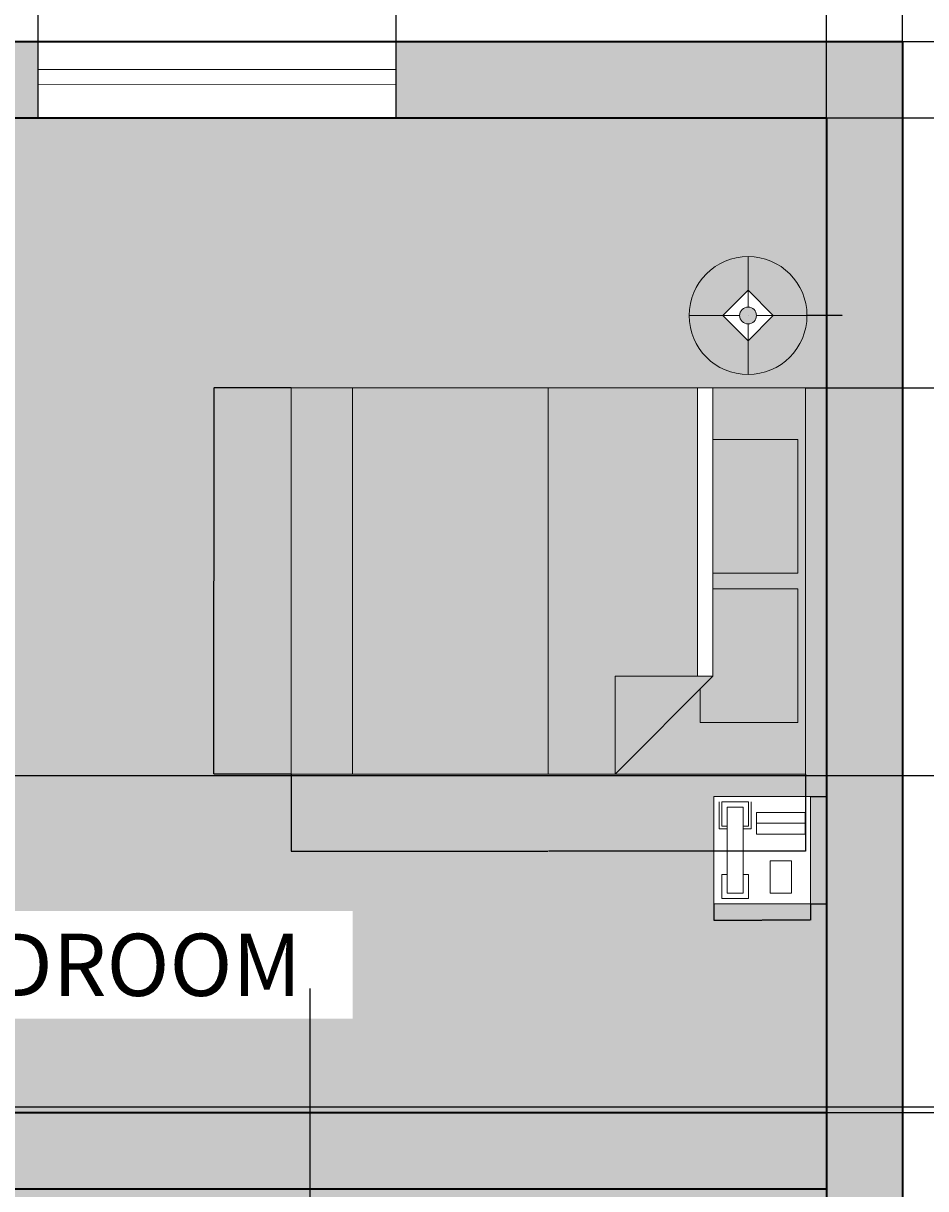
# Model space of a CAD drawing. Units: millimetres. Extents: x -229 to 16545, y -10488 to 4272.
# Tile 27 of 29: x 11362 to 14086, y -1208 to 2307. Entities that reach past the tile are written whole.
import ezdxf

# ---------------------------------------------------------------- set-up
doc = ezdxf.new("R2010")
doc.units = ezdxf.units.MM
for name, color, linetype, lineweight in [('A-ANNO-DIMS', 2, 'Continuous', 18), ('A-AREA-IDEN', 7, 'Continuous', 18), ('A-FURN', 8, 'Continuous', 18), ('A-FURN-PATT', 252, 'Continuous', 13), ('A-GLAZ', 4, 'Continuous', 18), ('A-WALL', 7, 'Continuous', 35)]:
    doc.layers.add(name, color=color, linetype=linetype, lineweight=lineweight)
doc.layers.add('A-FLOR-PATT', color=254, linetype='Continuous', lineweight=13, true_color=0xfeeab9)
doc.layers.add('A-WALL-PATT', color=18, linetype='Continuous', lineweight=13, true_color=0x000000)
doc.styles.get("Standard").update_dxf_attribs({"font": 'arial.ttf'})
doc.dimstyles.get("Standard").update_dxf_attribs({"dimtxt": 0.18, "dimasz": 0.18, "dimexe": 0.18, "dimexo": 0.0625, "dimgap": 0.09, "dimtad": 0, "dimtih": 1, "dimtoh": 1, "dimdec": 4, "dimzin": 0, "dimdsep": 46, "dimtxsty": 'Standard', "dimcen": 0.09, "dimadec": 0, "dimazin": 0, "dimtfac": 1, "dimtdec": 4, "dimtofl": 0, "dimtmove": 0, "dimatfit": 3, "dimfxl": 1, "dimtolj": 1, "dimtzin": 0, "dimarcsym": 0})

# ---------------------------------------------------------------- blocks, each defined once
blk = doc.blocks.new('Bed - Queen')
for p, q in [((0, -80.00003), (0, 0)), ((0, 0), (59.99999, 0)), ((59.99999, 0), (59.99999, -80.00003)), ((7.99999, -1.2), (28.79998, -1.2)), ((7.99999, -14.4), (7.99999, -1.2)), ((28.79998, -1.2), (28.79998, -14.4)), ((31.19999, -1.2), (51.99999, -1.2)), ((31.19999, -14.4), (31.19999, -1.2)), ((51.99999, -1.2), (51.99999, -16.4)), ((0, -14.4), (44.8, -14.4)), ((59.99999, -29.6), (44.8, -14.4)), ((44.8, -14.4), (44.8, -29.6)), ((44.8, -16.8), (0, -16.8)), ((51.99999, -16.4), (46.79936, -16.4)), ((44.8, -29.6), (59.99999, -29.6)), ((59.99999, -80.00003), (0, -80.00003))]:
    blk.add_line(p, q)
blk = doc.blocks.new('Lamp - Table')
for p, q in [((0, 7), (0, 1)), ((0, 3), (-3, 0)), ((3, 0), (0, 3)), ((-1, 0), (-7, 0)), ((-3, 0), (0, -3)), ((0, -3), (3, 0)), ((1, 0), (7, 0)), ((0, -1), (0, -7))]:
    blk.add_line(p, q)
for radius in [7, 1]:
    blk.add_circle((0, 0), radius)
blk = doc.blocks.new('Phone - Desk')
for p, q in [((-4.5, -5), (-4.5, 5)), ((-4.5, 5), (4.5, 5)), ((-4, 4.5), (-4, 2)), ((-3.75, 4.5), (-3.75, 2.25)), ((-1.25, 4.5), (-3.75, 4.5)), ((-1.25, 2.25), (-1.25, 4.5)), ((-1, 2), (-1, 4.5)), ((4.5, 5), (4.5, -5)), ((-3.25, 4), (-3.25, -4)), ((-3.25, 4), (-1.75, 4)), ((-1.75, -4), (-1.75, 4)), ((4, 3.5), (-0.5, 3.5)), ((-0.5, 3.5), (-0.5, 1.5)), ((4, 1.5), (4, 3.5)), ((-3.75, 2.25), (-3.25, 2.25)), ((-1.75, 2.25), (-1.25, 2.25)), ((-0.5, 2.5), (4, 2.5)), ((-4, 2), (-3.25, 2)), ((-1.75, 2), (-1, 2)), ((-0.5, 1.5), (4, 1.5)), ((2.75, -1), (0.75, -1)), ((0.75, -1), (0.75, -4)), ((2.75, -4), (2.75, -1)), ((-3.75, -2.25), (-3.25, -2.25)), ((-3.75, -4.5), (-3.75, -2.25)), ((-1.75, -2.25), (-1.25, -2.25)), ((-1.25, -2.25), (-1.25, -4.5)), ((-3.25, -4), (-1.75, -4)), ((0.75, -4), (2.75, -4)), ((4.5, -5), (-4.5, -5)), ((-1.25, -4.5), (-3.75, -4.5))]:
    blk.add_line(p, q)
blk = doc.blocks.new('*D31')
at = {"layer": 'A-ANNO-DIMS', "color": 0, "lineweight": -2, "transparency": 16777216}
for p, q in [((12170.5, 42.3), (12170.5, -190.7)), ((13722.9, 42.3), (13722.9, -190.7)), ((12170.6, -190.5), (12945.5, -190.5)), ((13722.7, -190.5), (12947.8, -190.5))]:
    blk.add_line(p, q, dxfattribs=at)
at = {"layer": 'A-ANNO-DIMS', "color": 0, "transparency": 16777216}
for points in [[(12170.6, -190.5), (12170.6, -190.5), (12170.5, -190.5)], [(13722.7, -190.5), (13722.7, -190.5), (13722.9, -190.5)]]:
    blk.add_solid(points, dxfattribs=at)
at = {"layer": 'Defpoints', "color": 0, "transparency": 16777216}
for p in [(12170.5, 42.4), (13722.9, 42.4), (13722.9, -190.5)]:
    blk.add_point(p, dxfattribs=at)
at = {"layer": 'A-ANNO-DIMS', "color": 0, "transparency": 16777216, "insert": (12946.7, -190.5), "char_height": 0.18, "attachment_point": 5}
blk.add_mtext('\\A1;QUEEN BED 1552', dxfattribs=at)
blk = doc.blocks.new('*D32')
at = {"layer": 'A-ANNO-DIMS', "color": 0, "lineweight": -2, "transparency": 16777216}
for p, q in [((12170.4, 1206.7), (11937.4, 1206.7)), ((11937.6, 1206.5), (11937.6, 624.7)), ((11937.6, 42.6), (11937.6, 624.4)), ((12170.4, 42.4), (11937.4, 42.4))]:
    blk.add_line(p, q, dxfattribs=at)
at = {"layer": 'A-ANNO-DIMS', "color": 0, "transparency": 16777216}
for points in [[(11937.6, 1206.5), (11937.6, 1206.5), (11937.6, 1206.7)], [(11937.6, 42.6), (11937.6, 42.6), (11937.6, 42.4)]]:
    blk.add_solid(points, dxfattribs=at)
at = {"layer": 'Defpoints', "color": 0, "transparency": 16777216}
for p in [(12170.5, 1206.7), (11937.6, 42.4), (12170.5, 42.4)]:
    blk.add_point(p, dxfattribs=at)
at = {"layer": 'A-ANNO-DIMS', "color": 0, "transparency": 16777216, "insert": (11937.6, 624.5), "char_height": 0.18, "attachment_point": 5}
blk.add_mtext('\\A1;1164', dxfattribs=at)
blk = doc.blocks.new('*D33')
at = {"layer": 'A-ANNO-DIMS', "color": 0, "lineweight": -2, "transparency": 16777216}
for p, q in [((13737.9, -25.2), (13786.6, -25.2)), ((13786.5, -25.4), (13786.5, -187.2)), ((13786.5, -349.4), (13786.5, -187.6)), ((13737.9, -349.6), (13786.6, -349.6))]:
    blk.add_line(p, q, dxfattribs=at)
at = {"layer": 'A-ANNO-DIMS', "color": 0, "transparency": 16777216}
for points in [[(13786.4, -25.4), (13786.5, -25.4), (13786.5, -25.2)], [(13786.4, -349.4), (13786.5, -349.4), (13786.5, -349.6)]]:
    blk.add_solid(points, dxfattribs=at)
at = {"layer": 'Defpoints', "color": 0, "transparency": 16777216}
for p in [(13737.8, -25.2), (13786.5, -25.2), (13737.8, -349.6)]:
    blk.add_point(p, dxfattribs=at)
at = {"layer": 'A-ANNO-DIMS', "color": 0, "transparency": 16777216, "insert": (13786.5, -187.4), "char_height": 0.18, "attachment_point": 5}
blk.add_mtext('\\A1;PHONE 324', dxfattribs=at)
blk = doc.blocks.new('*D34')
at = {"layer": 'A-ANNO-DIMS', "color": 0, "lineweight": -2, "transparency": 16777216}
for p, q in [((13445.9, -349.6), (13445.9, -398.4)), ((13737.8, -349.6), (13737.8, -398.4)), ((13446.1, -398.2), (13591.6, -398.2)), ((13737.6, -398.2), (13592.1, -398.2))]:
    blk.add_line(p, q, dxfattribs=at)
at = {"layer": 'A-ANNO-DIMS', "color": 0, "transparency": 16777216}
for points in [[(13446.1, -398.2), (13446.1, -398.3), (13445.9, -398.2)], [(13737.6, -398.2), (13737.6, -398.3), (13737.8, -398.2)]]:
    blk.add_solid(points, dxfattribs=at)
at = {"layer": 'Defpoints', "color": 0, "transparency": 16777216}
for p in [(13445.9, -349.6), (13737.8, -349.6), (13737.8, -398.2)]:
    blk.add_point(p, dxfattribs=at)
at = {"layer": 'A-ANNO-DIMS', "color": 0, "transparency": 16777216, "insert": (13591.8, -398.2), "char_height": 0.18, "attachment_point": 5}
blk.add_mtext('\\A1;292', dxfattribs=at)
blk = doc.blocks.new('*D45')
at = {"layer": 'A-ANNO-DIMS', "color": 0, "lineweight": -2, "transparency": 16777216}
for p, q in [((2015.9, 2251.8), (2015.9, 4271.7)), ((2016.1, 4271.5), (8015.5, 4271.5)), ((14015.8, 4271.5), (8016.4, 4271.5)), ((14015.9, 2251.8), (14015.9, 4271.7))]:
    blk.add_line(p, q, dxfattribs=at)
at = {"layer": 'A-ANNO-DIMS', "color": 0, "transparency": 16777216}
for points in [[(2016.1, 4271.5), (2016.1, 4271.4), (2015.9, 4271.5)], [(14015.8, 4271.5), (14015.8, 4271.4), (14015.9, 4271.5)]]:
    blk.add_solid(points, dxfattribs=at)
at = {"layer": 'Defpoints', "color": 0, "transparency": 16777216}
for p in [(14015.9, 4271.5), (2015.9, 2251.7), (14015.9, 2251.7)]:
    blk.add_point(p, dxfattribs=at)
at = {"layer": 'A-ANNO-DIMS', "color": 0, "transparency": 16777216, "insert": (8015.9, 4271.5), "char_height": 0.18, "attachment_point": 5}
blk.add_mtext('\\A1;12000', dxfattribs=at)
blk = doc.blocks.new('*D48')
at = {"layer": 'A-ANNO-DIMS', "color": 0, "lineweight": -2, "transparency": 16777216}
for p, q in [((14016, 2251.7), (16544.5, 2251.7)), ((16544.3, 2251.5), (16544.3, -1593.1)), ((16544.3, -5438.1), (16544.3, -1593.5)), ((13786, -5438.3), (16544.5, -5438.3))]:
    blk.add_line(p, q, dxfattribs=at)
at = {"layer": 'A-ANNO-DIMS', "color": 0, "transparency": 16777216}
for points in [[(16544.3, 2251.5), (16544.4, 2251.5), (16544.3, 2251.7)], [(16544.3, -5438.1), (16544.4, -5438.1), (16544.3, -5438.3)]]:
    blk.add_solid(points, dxfattribs=at)
at = {"layer": 'Defpoints', "color": 0, "transparency": 16777216}
for p in [(14015.9, 2251.7), (13785.9, -5438.3), (16544.3, -5438.3)]:
    blk.add_point(p, dxfattribs=at)
at = {"layer": 'A-ANNO-DIMS', "color": 0, "transparency": 16777216, "insert": (16544.3, -1593.3), "char_height": 0.18, "attachment_point": 5}
blk.add_mtext('\\A1;7690', dxfattribs=at)
blk = doc.blocks.new('*D52')
at = {"layer": 'A-ANNO-DIMS', "color": 0, "lineweight": -2, "transparency": 16777216}
for p, q in [((9785.9, -978.2), (9785.9, 4271.7)), ((9786.1, 4271.5), (11785.6, 4271.5)), ((13785.8, 4271.5), (11786.3, 4271.5)), ((13785.9, -978.2), (13785.9, 4271.7))]:
    blk.add_line(p, q, dxfattribs=at)
at = {"layer": 'A-ANNO-DIMS', "color": 0, "transparency": 16777216}
for points in [[(9786.1, 4271.5), (9786.1, 4271.4), (9785.9, 4271.5)], [(13785.8, 4271.5), (13785.8, 4271.4), (13785.9, 4271.5)]]:
    blk.add_solid(points, dxfattribs=at)
at = {"layer": 'Defpoints', "color": 0, "transparency": 16777216}
for p in [(13785.9, 4271.5), (9785.9, -978.3), (13785.9, -978.3)]:
    blk.add_point(p, dxfattribs=at)
at = {"layer": 'A-ANNO-DIMS', "color": 0, "transparency": 16777216, "insert": (11785.9, 4271.5), "char_height": 0.18, "attachment_point": 5}
blk.add_mtext('\\A1;4000', dxfattribs=at)
blk = doc.blocks.new('*D65')
at = {"layer": 'A-ANNO-DIMS', "color": 0, "lineweight": -2, "transparency": 16777216}
for p, q in [((13786, 2021.7), (16544.5, 2021.7)), ((16544.3, 2021.5), (16544.3, 521.9)), ((16544.3, -978.1), (16544.3, 521.5)), ((13786, -978.3), (16544.5, -978.3))]:
    blk.add_line(p, q, dxfattribs=at)
at = {"layer": 'A-ANNO-DIMS', "color": 0, "transparency": 16777216}
for points in [[(16544.3, 2021.5), (16544.4, 2021.5), (16544.3, 2021.7)], [(16544.3, -978.1), (16544.4, -978.1), (16544.3, -978.3)]]:
    blk.add_solid(points, dxfattribs=at)
at = {"layer": 'Defpoints', "color": 0, "transparency": 16777216}
for p in [(13785.9, 2021.7), (13785.9, -978.3), (16544.3, -978.3)]:
    blk.add_point(p, dxfattribs=at)
at = {"layer": 'A-ANNO-DIMS', "color": 0, "transparency": 16777216, "insert": (16544.3, 521.7), "char_height": 0.18, "attachment_point": 5}
blk.add_mtext('\\A1;3000', dxfattribs=at)
blk = doc.blocks.new('*D66')
at = {"layer": 'A-ANNO-DIMS', "color": 0, "lineweight": -2, "transparency": 16777216}
for p, q in [((9556, 38.2), (16544.5, 38.2)), ((16544.3, 38), (16544.3, -461.6)), ((16544.3, -961.6), (16544.3, -462)), ((9556, -961.8), (16544.5, -961.8))]:
    blk.add_line(p, q, dxfattribs=at)
at = {"layer": 'A-ANNO-DIMS', "color": 0, "transparency": 16777216}
for points in [[(16544.3, 38), (16544.4, 38), (16544.3, 38.2)], [(16544.3, -961.6), (16544.4, -961.6), (16544.3, -961.8)]]:
    blk.add_solid(points, dxfattribs=at)
at = {"layer": 'Defpoints', "color": 0, "transparency": 16777216}
for p in [(9555.9, 38.2), (9555.9, -961.8), (16544.3, -961.8)]:
    blk.add_point(p, dxfattribs=at)
at = {"layer": 'A-ANNO-DIMS', "color": 0, "transparency": 16777216, "insert": (16544.3, -461.8), "char_height": 0.18, "attachment_point": 5}
blk.add_mtext('\\A1;1000', dxfattribs=at)
blk = doc.blocks.new('*D67')
at = {"layer": 'A-ANNO-DIMS', "color": 0, "lineweight": -2, "transparency": 16777216}
for p, q in [((11407.5, 2021.8), (11407.5, 4271.7)), ((11407.7, 4271.5), (11947.3, 4271.5)), ((12487.8, 4271.5), (11948.2, 4271.5)), ((12488, 2021.8), (12488, 4271.7))]:
    blk.add_line(p, q, dxfattribs=at)
at = {"layer": 'A-ANNO-DIMS', "color": 0, "transparency": 16777216}
for points in [[(11407.7, 4271.5), (11407.7, 4271.4), (11407.5, 4271.5)], [(12487.8, 4271.5), (12487.8, 4271.4), (12488, 4271.5)]]:
    blk.add_solid(points, dxfattribs=at)
at = {"layer": 'Defpoints', "color": 0, "transparency": 16777216}
for p in [(12488, 4271.5), (11407.5, 2021.7), (12488, 2021.7)]:
    blk.add_point(p, dxfattribs=at)
at = {"layer": 'A-ANNO-DIMS', "color": 0, "transparency": 16777216, "insert": (11947.8, 4271.5), "char_height": 0.18, "attachment_point": 5}
blk.add_mtext('\\A1;1080.5', dxfattribs=at)
blk = doc.blocks.new('*D68')
at = {"layer": 'A-ANNO-DIMS', "color": 0, "lineweight": -2, "transparency": 16777216}
for p, q in [((12488, 2021.8), (12488, 4271.7)), ((12488.2, 4271.5), (13136.6, 4271.5)), ((13785.8, 4271.5), (13137.3, 4271.5)), ((13785.9, 2021.8), (13785.9, 4271.7))]:
    blk.add_line(p, q, dxfattribs=at)
at = {"layer": 'A-ANNO-DIMS', "color": 0, "transparency": 16777216}
for points in [[(12488.2, 4271.5), (12488.2, 4271.4), (12488, 4271.5)], [(13785.8, 4271.5), (13785.8, 4271.4), (13785.9, 4271.5)]]:
    blk.add_solid(points, dxfattribs=at)
at = {"layer": 'Defpoints', "color": 0, "transparency": 16777216}
for p in [(13785.9, 4271.5), (12488, 2021.7), (13785.9, 2021.7)]:
    blk.add_point(p, dxfattribs=at)
at = {"layer": 'A-ANNO-DIMS', "color": 0, "transparency": 16777216, "insert": (13137, 4271.5), "char_height": 0.18, "attachment_point": 5}
blk.add_mtext('\\A1;1298', dxfattribs=at)
blk = doc.blocks.new('*D99')
at = {"layer": 'A-ANNO-DIMS', "color": 0, "lineweight": -2, "transparency": 16777216}
for p, q in [((13786, 2021.7), (16544.5, 2021.7)), ((16544.3, 2021.5), (16544.3, 1614.4)), ((16544.3, 1206.9), (16544.3, 1614)), ((13723, 1206.7), (16544.5, 1206.7))]:
    blk.add_line(p, q, dxfattribs=at)
at = {"layer": 'A-ANNO-DIMS', "color": 0, "transparency": 16777216}
for points in [[(16544.3, 2021.5), (16544.4, 2021.5), (16544.3, 2021.7)], [(16544.3, 1206.9), (16544.4, 1206.9), (16544.3, 1206.7)]]:
    blk.add_solid(points, dxfattribs=at)
at = {"layer": 'Defpoints', "color": 0, "transparency": 16777216}
for p in [(13785.9, 2021.7), (13722.9, 1206.7), (16544.3, 1206.7)]:
    blk.add_point(p, dxfattribs=at)
at = {"layer": 'A-ANNO-DIMS', "color": 0, "transparency": 16777216, "insert": (16544.3, 1614.2), "char_height": 0.18, "attachment_point": 5}
blk.add_mtext('\\A1;815', dxfattribs=at)
blk = doc.blocks.new('*D103')
at = {"layer": 'A-ANNO-DIMS', "color": 0, "lineweight": -2, "transparency": 16777216}
for p, q in [((12227, -604.2), (12226.8, -604.2)), ((12226.8, -604.2), (12226.8, -1372.9)), ((12226.7, -2654.6), (12226.9, -2654.6)), ((12226.8, -2654.7), (12226.8, -2654.5))]:
    blk.add_line(p, q, dxfattribs=at)
at = {"layer": 'A-ANNO-DIMS', "color": 0, "transparency": 16777216}
blk.add_solid([(12226.8, -1372.9), (12226.9, -1372.9), (12226.8, -1373.1)], dxfattribs=at)
at = {"layer": 'Defpoints', "color": 0, "transparency": 16777216}
for p in [(12226.8, -1373.1), (12226.8, -2654.6)]:
    blk.add_point(p, dxfattribs=at)
at = {"layer": 'A-ANNO-DIMS', "color": 0, "transparency": 16777216, "insert": (12227.6, -604.2), "char_height": 0.18, "attachment_point": 5}
blk.add_mtext('\\A1;R1281.5', dxfattribs=at)
blk = doc.blocks.new('*D104')
at = {"layer": 'A-ANNO-DIMS', "color": 0, "lineweight": -2, "transparency": 16777216}
for p, q in [((12227, -793.9), (12226.8, -793.9)), ((12226.8, -793.9), (12226.8, -1500.5)), ((12226.7, -2678.7), (12226.9, -2678.7)), ((12226.8, -2678.8), (12226.8, -2678.6))]:
    blk.add_line(p, q, dxfattribs=at)
at = {"layer": 'A-ANNO-DIMS', "color": 0, "transparency": 16777216}
blk.add_solid([(12226.8, -1500.5), (12226.9, -1500.5), (12226.8, -1500.7)], dxfattribs=at)
at = {"layer": 'Defpoints', "color": 0, "transparency": 16777216}
for p in [(12226.8, -1500.7), (12226.8, -2678.7)]:
    blk.add_point(p, dxfattribs=at)
at = {"layer": 'A-ANNO-DIMS', "color": 0, "transparency": 16777216, "insert": (12227.5, -793.9), "char_height": 0.18, "attachment_point": 5}
blk.add_mtext('\\A1;R1178', dxfattribs=at)
blk = doc.blocks.new('*D106')
at = {"layer": 'A-ANNO-DIMS', "color": 0, "lineweight": -2, "transparency": 16777216}
for p, q in [((13549.6, 1425.2), (13549.8, 1425.2)), ((13549.7, 1425.1), (13549.7, 1425.3)), ((13834.1, 1425.2), (13727.6, 1425.2))]:
    blk.add_line(p, q, dxfattribs=at)
at = {"layer": 'A-ANNO-DIMS', "color": 0, "transparency": 16777216}
blk.add_solid([(13727.6, 1425.2), (13727.6, 1425.2), (13727.5, 1425.2)], dxfattribs=at)
at = {"layer": 'Defpoints', "color": 0, "transparency": 16777216}
for p in [(13371.9, 1425.2), (13727.5, 1425.2)]:
    blk.add_point(p, dxfattribs=at)
at = {"layer": 'A-ANNO-DIMS', "color": 0, "transparency": 16777216, "insert": (13834.8, 1425.2), "char_height": 0.18, "attachment_point": 5}
blk.add_mtext('\\A1;2X ∅355.6', dxfattribs=at)

msp = doc.modelspace()

# ---------------------------------------------------------------- hatches: boundary and pattern name
at = {"layer": 'A-FLOR-PATT', "transparency": 33554592}
h = msp.add_hatch(color=256, dxfattribs=at)
h.dxf.hatch_style = 1
h.paths.add_polyline_path([(7975.933, -5325.772), (7943.121, -5325.772), (7943.121, -4576.49, 0.40145271), (7225.933, -5325.772, 0.40145271), (6508.746, -4576.49), (6508.746, -5325.772), (6475.933, -5325.772), (6475.933, -5438.272), (5975.933, -5438.272), (5975.933, -7267.724), (5975.933, -7438.272), (6478.619, -7438.272), (6463.448, -7355.919), (6464.88, -7356.837), (6463.849, -7358.097), (6478.619, -7438.272), (6610.327, -7438.272), (6632.656, -7409.564), (6632.525, -7406.967), (6634.208, -7407.569), (6619.273, -7426.77), (6654.466, -7438.272), (7610.517, -7438.272), (7607.41, -7421.409), (7608.842, -7422.327), (7607.812, -7423.587), (7610.517, -7438.272), (7975.933, -7438.272)])
h.paths.add_polyline_path([(13785.933, -1208.272), (9555.933, -1208.272), (9555.933, -961.785), (9705.933, -961.785), (9705.933, -918.035), (10704.976, -918.035, 0.40145271), (9705.933, 38.215), (9555.933, 38.215), (9555.933, 2021.728), (5975.933, 2021.728), (5975.933, 755.492), (5745.933, 755.492), (5745.933, 1427.266), (2918.813, 1427.266), (2918.813, -492.942), (5013.319, -492.942), (5013.319, -978.272), (5745.933, -978.272), (5745.933, -397.513), (5975.933, -397.513), (5975.933, -1208.272), (4560.933, -1208.272), (4560.933, -1265.772), (4448.433, -1265.772), (4448.433, -1298.585), (4445.933, -1298.585), (3699.151, -1298.585, 0.40145271), (4448.433, -2015.772), (4560.933, -2015.772), (4560.933, -2384.177), (5745.933, -2384.177), (5799.402, -2384.177), (5799.402, -4518.272), (5975.933, -4518.272), (5975.933, -5208.272), (6475.933, -5208.272), (6475.933, -4575.772), (6508.746, -4575.772), (6508.746, -4576.49, -0.35647263), (7216.672, -5208.272), (7235.194, -5208.272, -0.35647263), (7943.121, -4576.49), (7943.121, -4575.772), (7975.933, -4575.772), (7975.933, -5208.272), (11176.247, -5208.272), (11159.44, -5191.465), (10520.768, -5191.465), (10520.768, -4888.936), (10571.19, -4888.936), (10571.19, -4872.129), (10772.876, -4872.129), (10772.876, -4888.936), (10789.683, -4888.936), (10789.683, -4872.129), (10991.368, -4872.129), (10991.368, -4888.936), (11041.79, -4888.936), (11041.79, -4872.129), (11058.597, -4872.129, -0.09090909), (11428.354, -4872.129), (11445.162, -4872.129), (11445.162, -4888.936), (11529.197, -4888.936), (11529.197, -5191.465), (11327.512, -5191.465), (11310.704, -5208.272), (13785.933, -5208.272)])
h.paths.add_polyline_path([(11047.216, -1630.944, -1), (11402.816, -1630.944, -1)], flags=16)
h.paths.add_polyline_path([(11148.816, -1630.944), (11225.016, -1554.744), (11301.216, -1630.944), (11225.016, -1707.144)], flags=0)
h.paths.add_polyline_path([(11199.616, -1630.944, -1), (11250.416, -1630.944, -1)], flags=0)
h.paths.add_polyline_path([(11588.751, -2096.259), (11588.751, -1543.254, -0.26666697), (12864.918, -1543.254), (12864.918, -2096.259), (12737.302, -2096.259), (12737.302, -2063.121), (11716.368, -2063.121), (11716.368, -2096.259)], flags=16)
h.paths.add_polyline_path([(12012.696, -2489.42), (12600.997, -2489.42), (12600.997, -3666.022), (12012.696, -3666.022)], flags=16)
h.paths.add_polyline_path([(12176.41, -3599.403), (12174.938, -3609.076), (12173.789, -3618.819), (12173.09, -3628.559), (12172.973, -3638.221), (12173.89, -3652.852), (12175.008, -3657.025), (12172.909, -3643.473), (12173.142, -3624.297), (12175.386, -3605.273)], flags=0)
h.paths.add_polyline_path([(8026.289, -286.944), (7737.703, -287.19), (7734.87, -269.156), (8029.092, -268.905)], flags=16)
h.paths.add_polyline_path([(7733.453, -260.139), (7710.784, -115.865), (7557.191, -115.996), (7556.999, 109.744), (7412.687, 132.166), (7412.433, 429.206), (7556.707, 451.876), (7556.568, 614.769), (7412.256, 637.19), (7412.003, 934.231), (7556.276, 956.9), (7556.084, 1182.639), (7709.677, 1182.77), (7732.099, 1327.082), (8029.14, 1327.335), (8051.808, 1183.062), (8205.401, 1183.192), (8205.594, 957.454), (8349.906, 935.031), (8350.159, 637.99), (8205.885, 615.322), (8206.024, 452.43), (8350.336, 430.006), (8350.59, 132.965), (8206.316, 110.298), (8206.509, -115.442), (8052.916, -115.573), (8030.493, -259.885)], flags=16)
h.paths.add_polyline_path([(12261.416, -3475.554), (12262.632, -3486.776), (12264.032, -3497.007), (12265.554, -3506.365), (12267.136, -3514.968), (12268.719, -3522.935), (12271.304, -3535.59), (12273.606, -3548.078), (12275.271, -3561.064), (12275.93, -3574.938), (12275.325, -3590.3), (12273.425, -3607.964), (12270.795, -3625.658), (12268.066, -3641.063), (12266.318, -3649.679), (12265.456, -3653.626), (12263.984, -3659.846), (12264.032, -3659.566), (12264.342, -3658.241), (12264.807, -3656.37), (12265.456, -3653.626), (12266.318, -3649.679), (12267.409, -3644.302), (12268.668, -3637.664), (12270.019, -3630.037), (12271.384, -3621.695), (12272.69, -3612.908), (12273.857, -3603.948), (12274.81, -3595.088), (12275.47, -3586.601), (12275.782, -3578.689), (12275.757, -3571.292), (12275.423, -3564.275), (12274.816, -3557.512), (12273.964, -3550.872), (12272.896, -3544.224), (12271.645, -3537.439), (12270.24, -3530.385), (12267.543, -3517.181), (12264.612, -3501.247), (12261.849, -3481.059)], flags=0)
h.paths.add_polyline_path([(12332.136, -3408.03), (12333.483, -3416.79), (12335.077, -3424.54), (12336.915, -3431.355), (12338.991, -3437.32), (12341.266, -3442.55), (12343.694, -3447.166), (12346.229, -3451.292), (12348.826, -3455.051), (12351.438, -3458.563), (12357.476, -3466.491), (12363.61, -3476.575), (12368.309, -3489.762), (12369.929, -3503.427), (12369.842, -3516.511), (12368.43, -3530.867), (12365.816, -3545.835), (12362.382, -3559.786), (12360.968, -3564.487), (12363.063, -3557.021), (12364.898, -3549.566), (12366.473, -3542.077), (12367.773, -3534.631), (12368.781, -3527.301), (12369.483, -3520.162), (12369.863, -3513.291), (12369.906, -3506.759), (12369.599, -3500.643), (12368.93, -3494.999), (12367.924, -3489.796), (12366.61, -3484.994), (12365.024, -3480.542), (12363.19, -3476.399), (12361.141, -3472.516), (12358.909, -3468.847), (12356.525, -3465.347), (12354.02, -3461.954), (12351.438, -3458.563), (12345.462, -3450.529), (12339.923, -3439.996), (12335.85, -3428.296), (12332.68, -3412.888)], flags=0)
h.paths.add_polyline_path([(12385.287, -3334.612), (12384.977, -3342.409), (12385.02, -3349.196), (12385.4, -3355.066), (12386.104, -3360.105), (12387.112, -3364.41), (12388.412, -3368.071), (12389.987, -3371.181), (12391.823, -3373.832), (12393.919, -3376.097), (12396.337, -3377.978), (12399.153, -3379.462), (12402.445, -3380.531), (12406.289, -3381.172), (12410.758, -3381.371), (12415.935, -3381.106), (12421.893, -3380.368), (12428.658, -3379.159), (12436.069, -3377.55), (12443.907, -3375.635), (12451.961, -3373.505), (12460.015, -3371.254), (12467.853, -3368.971), (12475.263, -3366.749), (12482.029, -3364.68), (12491.877, -3361.657), (12497.701, -3360.107), (12501.639, -3359.288), (12510.135, -3358.326), (12519.662, -3365.412), (12524.243, -3378.911), (12523.764, -3390.7), (12520.746, -3401.577), (12514.248, -3415.634), (12511.518, -3420.418), (12515.856, -3412.154), (12519.153, -3405.024), (12521.516, -3398.804), (12523.049, -3393.276), (12523.865, -3388.212), (12524.059, -3383.441), (12523.7, -3378.958), (12522.853, -3374.815), (12521.576, -3371.054), (12519.931, -3367.722), (12517.982, -3364.865), (12515.786, -3362.529), (12513.405, -3360.758), (12510.877, -3359.588), (12508.136, -3358.982), (12505.086, -3358.897), (12501.639, -3359.288), (12497.701, -3360.107), (12493.183, -3361.309), (12487.988, -3362.851), (12476.403, -3366.408), (12463.335, -3370.326), (12447.372, -3374.788), (12431.759, -3378.604), (12418.504, -3380.974), (12405.811, -3381.624), (12394.725, -3378.025), (12388.039, -3368.367), (12385.583, -3357.877), (12384.826, -3346.204), (12385.428, -3331.059), (12385.953, -3325.719)], flags=0)
h.paths.add_polyline_path([(7880.016, 1173.969), (7880.373, 1175.495), (7880.433, 1175.851), (7879.484, 1171.818)], flags=0)
h.paths.add_polyline_path([(7802.33, 874.962), (7800.771, 885.032), (7798.932, 893.941), (7796.811, 901.774), (7794.419, 908.63), (7791.798, 914.639), (7789.002, 919.945), (7786.083, 924.686), (7783.093, 929.005), (7780.087, 933.043), (7774.996, 939.717), (7768.406, 949.37), (7762.174, 963.427), (7759.342, 978.002), (7758.629, 991.888), (7759.492, 1007.928), (7761.801, 1025.496), (7765.392, 1044.035), (7766.625, 1049.048), (7764.522, 1039.543), (7762.719, 1030.232), (7761.232, 1021.168), (7760.08, 1012.405), (7759.28, 1003.994), (7758.849, 995.988), (7758.806, 988.44), (7759.167, 981.404), (7759.942, 974.914), (7761.104, 968.936), (7762.617, 963.414), (7764.448, 958.299), (7766.559, 953.535), (7768.918, 949.073), (7771.487, 944.856), (7774.232, 940.835), (7777.115, 936.938), (7782.377, 930.041), (7787.845, 922.139), (7793.348, 911.698), (7798.042, 898.247), (7801.702, 880.527)], flags=0)
h.paths.add_polyline_path([(12519.068, -3228.534), (12519.615, -3236.235), (12520.529, -3242.343), (12521.78, -3247.103), (12523.337, -3250.758), (12525.171, -3253.556), (12527.248, -3255.709), (12529.522, -3257.296), (12531.95, -3258.361), (12534.486, -3258.949), (12537.082, -3259.11), (12539.694, -3258.888), (12542.277, -3258.329), (12544.781, -3257.478), (12547.173, -3256.388), (12549.46, -3255.129), (12550.455, -3254.517), (12555.825, -3251.109), (12557.835, -3249.942), (12565.181, -3246.404), (12574.565, -3253.032), (12576.931, -3265.022), (12576.627, -3277.425), (12575.416, -3290.819), (12574.851, -3295.392), (12575.708, -3287.593), (12576.322, -3280.806), (12576.688, -3274.939), (12576.812, -3269.899), (12576.688, -3265.593), (12576.322, -3261.932), (12575.708, -3258.822), (12574.851, -3256.172), (12573.753, -3253.905), (12572.439, -3252.005), (12570.943, -3250.474), (12569.293, -3249.309), (12567.523, -3248.513), (12565.658, -3248.083), (12563.732, -3248.022), (12561.777, -3248.328), (12559.814, -3248.989), (12557.835, -3249.942), (12555.825, -3251.109), (12553.77, -3252.413), (12551.652, -3253.78), (12549.46, -3255.129), (12543.167, -3258.594), (12532.661, -3259.485), (12524.685, -3253.923), (12520.949, -3245.152), (12519.138, -3233.042)], flags=0)
h.paths.add_polyline_path([(7741.293, 790.501), (7741.641, 799.467), (7741.584, 807.269), (7741.141, 814.015), (7740.329, 819.809), (7739.165, 824.757), (7737.667, 828.966), (7735.853, 832.541), (7733.74, 835.586), (7731.348, 838.188), (7728.71, 840.348), (7725.861, 842.052), (7722.836, 843.28), (7719.671, 844.015), (7716.4, 844.237), (7713.06, 843.932), (7709.684, 843.081), (7706.304, 841.686), (7702.923, 839.834), (7699.543, 837.629), (7696.164, 835.178), (7692.784, 832.585), (7684.718, 826.315), (7675.609, 820.63), (7664.001, 817.274), (7654.105, 821.884), (7647.171, 832.02), (7644.191, 846.522), (7646.321, 860.288), (7647.49, 864.223), (7645.946, 857.865), (7645.046, 852.044), (7644.827, 846.557), (7645.243, 841.404), (7646.221, 836.642), (7647.693, 832.318), (7649.587, 828.489), (7651.832, 825.206), (7654.359, 822.523), (7657.097, 820.49), (7659.984, 819.145), (7662.993, 818.452), (7666.108, 818.357), (7669.311, 818.809), (7672.583, 819.755), (7675.908, 821.139), (7679.268, 822.913), (7682.645, 825.021), (7686.025, 827.401), (7689.404, 829.958), (7692.784, 832.585), (7700.505, 838.509), (7709.871, 843.64), (7721.436, 844.698), (7733.277, 837.617), (7739.571, 825.214), (7741.557, 811.049), (7741.669, 795.575)], flags=0)
h.paths.add_polyline_path([(8377.641, 137.216), (8359.607, 134.382), (8359.356, 428.605), (8377.395, 425.802)], flags=16)
h.paths.add_polyline_path([(7650.715, 668.465), (7650.08, 677.319), (7649.023, 684.34), (7647.579, 689.811), (7645.785, 694.012), (7643.675, 697.228), (7641.286, 699.7), (7638.669, 701.521), (7635.876, 702.744), (7632.96, 703.419), (7629.974, 703.601), (7626.971, 703.344), (7624.004, 702.697), (7621.125, 701.717), (7618.375, 700.462), (7615.749, 699.013), (7614.561, 698.279), (7608.435, 694.382), (7606.125, 693.04), (7598.981, 689.594), (7589.669, 693.773), (7585.26, 702.856), (7584.221, 713.11), (7584.49, 724.584), (7585.863, 739.937), (7586.518, 745.277), (7585.539, 736.31), (7584.841, 728.507), (7584.424, 721.761), (7584.288, 715.966), (7584.433, 711.016), (7584.86, 706.807), (7585.567, 703.231), (7586.556, 700.186), (7587.821, 697.58), (7589.332, 695.397), (7591.053, 693.637), (7592.951, 692.3), (7594.989, 691.385), (7597.132, 690.895), (7599.346, 690.826), (7601.594, 691.18), (7603.851, 691.943), (7606.125, 693.04), (7608.435, 694.382), (7610.797, 695.885), (7613.229, 697.458), (7620.475, 701.929), (7632.001, 704.44), (7643.476, 699.417), (7648.536, 687.571), (7650.63, 673.661)], flags=0)
h.paths.add_polyline_path([(7385.628, 136.37), (7385.382, 424.956), (7403.416, 427.789), (7403.667, 133.567)], flags=16)
h.paths.add_polyline_path([(12993.884, -2257.186), (12959.588, -2257.186), (12959.588, -2125.099), (13531.966, -2125.099, -0.19047621), (13531.966, -3974.321), (12959.588, -3974.321), (12959.588, -3842.233), (12993.884, -3842.233)], flags=16)
h.paths.add_polyline_path([(13413.486, -3313.884), (13413.486, -2785.535), (13562.885, -2785.535, -0.04962821), (13562.885, -3313.884)], flags=0)
h.paths.add_polyline_path([(8377.21, 642.241), (8359.176, 639.407), (8358.925, 933.629), (8376.964, 930.826)], flags=16)
h.paths.add_polyline_path([(13086.058, -1864.83), (13086.058, -1449.84), (13501.048, -1449.84), (13501.048, -1864.83)], flags=16)
h.paths.add_polyline_path([(13305.814, -1862.197), (13302.103, -1859.624), (13298.088, -1857.068), (13293.799, -1854.536), (13289.262, -1852.031), (13284.504, -1849.559), (13279.554, -1847.125), (13274.439, -1844.735), (13269.17, -1842.389), (13263.701, -1840.081), (13257.97, -1837.797), (13251.914, -1835.525), (13245.472, -1833.252), (13238.582, -1830.968), (13231.18, -1828.66), (13223.206, -1826.315), (13209.182, -1822.458), (13204.584, -1821.48), (13217.962, -1824.773), (13235.072, -1829.804), (13248.777, -1834.349), (13260.829, -1838.869), (13274.479, -1844.63), (13289.675, -1852.101), (13302.553, -1859.704)], flags=0)
h.paths.add_polyline_path([(13428.104, -1820.994), (13419.007, -1818.141), (13409.95, -1815.4), (13400.766, -1812.747), (13391.271, -1810.151), (13376.087, -1806.251), (13370.618, -1805.019), (13386.304, -1808.794), (13405.087, -1813.928), (13423.014, -1819.354)], flags=0)
h.paths.add_polyline_path([(7385.197, 641.395), (7384.951, 929.98), (7402.986, 932.814), (7403.236, 638.592)], flags=16)
h.paths.add_polyline_path([(13262.537, -1725.526), (13253.246, -1724.74), (13244.516, -1724.117), (13235.94, -1723.625), (13223.267, -1723.062), (13217.598, -1722.912), (13231.966, -1723.397), (13248.733, -1724.359), (13266.899, -1725.895), (13272.802, -1726.502)], flags=0)
h.paths.add_polyline_path([(13191.893, -1641.137), (13208.675, -1640.506), (13214.057, -1640.258), (13197.763, -1640.936)], flags=0)
h.paths.add_polyline_path([(13097.524, -1608.457), (13114.284, -1609.031), (13120.126, -1609.105), (13103.045, -1608.71)], flags=0)
h.paths.add_polyline_path([(13465.328, -1521.577), (13473.906, -1517.015), (13481.761, -1511.636), (13492.562, -1502.076), (13495.327, -1497.933), (13485.818, -1508.858), (13470.208, -1519.547)], flags=0)
h.paths.add_polyline_path([(13175.015, -1500.891), (13184.046, -1501.807), (13192.721, -1502.52), (13201.114, -1503.034), (13209.273, -1503.351), (13217.244, -1503.476), (13225.078, -1503.41), (13232.821, -1503.16), (13240.524, -1502.728), (13248.233, -1502.117), (13255.993, -1501.322), (13263.825, -1500.293), (13271.746, -1498.974), (13279.775, -1497.305), (13287.928, -1495.229), (13296.222, -1492.688), (13304.675, -1489.622), (13313.304, -1485.975), (13322.089, -1481.727), (13330.859, -1477.028), (13339.408, -1472.063), (13347.526, -1467.02), (13355.006, -1462.087), (13364.86, -1455.202), (13367.224, -1453.299), (13358.544, -1459.754), (13343.348, -1469.775), (13326.143, -1479.767), (13309.023, -1488.045), (13292.249, -1494.129), (13276.009, -1498.264), (13260.299, -1500.88), (13244.401, -1502.51), (13228.945, -1503.378), (13213.316, -1503.508), (13197.047, -1502.876), (13180.088, -1501.481)], flags=0)
h.paths.add_polyline_path([(7733.501, 1336.101), (7736.303, 1354.14), (8024.889, 1354.386), (8027.723, 1336.352)], flags=16)
h = msp.add_hatch(color=256, dxfattribs=at)
h.dxf.hatch_style = 1
h.paths.add_polyline_path([(13785.933, 2021.728), (9555.933, 2021.728), (9555.933, 38.215), (9705.933, 38.215, -0.40145271), (10704.976, -918.035), (10705.933, -918.035), (10705.933, -978.272), (13785.933, -978.272)])
h.paths.add_polyline_path([(12170.451, 1206.716), (13722.905, 1206.716), (13722.905, 42.377), (12170.451, 42.377)], flags=16)
h.paths.add_polyline_path([(10122.076, 374.936), (10105.269, 374.936), (10105.269, 290.901), (9802.74, 290.901), (9802.74, 492.586), (9785.933, 509.394), (9785.933, 643.851), (9802.74, 660.658), (9802.74, 1299.33), (10105.269, 1299.33), (10105.269, 1248.908), (10122.076, 1248.908), (10122.076, 1047.222), (10105.269, 1047.222), (10105.269, 1030.415), (10122.076, 1030.415), (10122.076, 828.729), (10105.269, 828.729), (10105.269, 778.308), (10122.076, 778.308), (10122.076, 761.501, -0.09090909), (10122.076, 391.743)], flags=16)
h.paths.add_polyline_path([(10096.865, 299.304), (9811.144, 299.304), (9811.144, 1290.926), (10096.865, 1290.926)], flags=0)
h.paths.add_polyline_path([(13148.497, 337.342), (13443.463, 337.342), (13443.463, 1051.471), (13699.618, 1051.471), (13699.618, 647.833), (13443.463, 647.833), (13443.463, 601.26), (13699.618, 601.26), (13699.618, 197.622), (13404.652, 197.622), (13404.652, 298.531), (13148.497, 42.377)], flags=0)
h.paths.add_polyline_path([(13445.876, -25.215), (13737.804, -25.215), (13737.804, -349.58), (13445.876, -349.58)], flags=16)
h.paths.add_polyline_path([(13462.094, -41.433), (13559.404, -41.433), (13559.404, -122.524), (13535.076, -122.524), (13535.076, -260.379), (13551.295, -260.379), (13551.295, -333.361), (13470.203, -333.361), (13470.203, -260.379), (13486.422, -260.379), (13486.422, -122.524), (13462.094, -122.524)], flags=0)
h.paths.add_polyline_path([(13575.622, -73.869), (13721.586, -73.869), (13721.586, -138.742), (13575.622, -138.742)], flags=0)
h.paths.add_polyline_path([(13616.168, -219.834), (13681.04, -219.834), (13681.04, -317.143), (13616.168, -317.143)], flags=0)
h.paths.add_polyline_path([(13371.868, 1425.214, -1), (13727.468, 1425.214, -1)], flags=16)
h.paths.add_polyline_path([(13473.468, 1425.214), (13549.668, 1501.414), (13625.868, 1425.214), (13549.668, 1349.014)], flags=0)
h.paths.add_polyline_path([(13524.268, 1425.214, -1), (13575.068, 1425.214, -1)], flags=0)
at = {"layer": 'A-FURN-PATT'}
h = msp.add_hatch(color=256, dxfattribs=at)
h.dxf.hatch_style = 1
h.paths.add_polyline_path([(13549.668, 1603.014, 0.41421356), (13371.868, 1425.214), (13473.468, 1425.214), (13549.668, 1501.414)])
h.paths.add_polyline_path([(13549.668, 1603.014), (13549.668, 1501.414), (13625.868, 1425.214), (13727.468, 1425.214, 0.41421356)])
h.paths.add_polyline_path([(13727.468, 1425.214), (13625.868, 1425.214), (13549.668, 1349.014), (13549.668, 1247.414, 0.41421356)])
h.paths.add_polyline_path([(13473.468, 1425.214), (13371.868, 1425.214, 0.41421356), (13549.668, 1247.414), (13549.668, 1349.014)])
h.paths.add_polyline_path([(13524.268, 1425.214, 1), (13575.068, 1425.214, 1)])
h.paths.add_polyline_path([(11148.816, -1630.944), (11047.216, -1630.944, 0.41421356), (11225.016, -1808.744), (11225.016, -1707.144)])
h.paths.add_polyline_path([(11402.816, -1630.944), (11301.216, -1630.944), (11225.016, -1707.144), (11225.016, -1808.744, 0.41421356)])
h.paths.add_polyline_path([(11225.016, -1453.144, 0.41421356), (11047.216, -1630.944), (11148.816, -1630.944), (11225.016, -1554.744)])
h.paths.add_polyline_path([(11225.016, -1453.144), (11225.016, -1554.744), (11301.216, -1630.944), (11402.816, -1630.944, 0.41421356)])
h.paths.add_polyline_path([(11199.616, -1630.944, 1), (11250.416, -1630.944, 1)])
h = msp.add_hatch(color=256, dxfattribs=at)
h.dxf.hatch_style = 1
h.paths.add_polyline_path([(12355.769, 1206.716), (12170.451, 1206.716), (12170.451, 42.377), (12355.769, 42.377)])
h.paths.add_polyline_path([(13396.89, 1206.716), (12946.678, 1206.716), (12946.678, 42.377), (13148.497, 42.377), (13148.497, 337.342), (13396.89, 337.342)])
h.paths.add_polyline_path([(13722.905, 1206.716), (13443.463, 1206.716), (13443.463, 1051.471), (13699.618, 1051.471), (13699.618, 647.833), (13443.463, 647.833), (13443.463, 601.26), (13699.618, 601.26), (13699.618, 197.622), (13404.652, 197.622), (13404.652, 298.531), (13148.497, 42.377), (13722.905, 42.377)])
at = {"layer": 'A-FURN-PATT', "transparency": 33554646}
h = msp.add_hatch(color=256, dxfattribs=at)
h.dxf.hatch_style = 1
h.paths.add_polyline_path([(12946.678, 1206.716), (12355.769, 1206.716), (12355.769, 42.377), (12946.678, 42.377)])
h.paths.add_polyline_path([(13699.618, 1051.471), (13443.463, 1051.471), (13443.463, 647.833), (13699.618, 647.833)])
h.paths.add_polyline_path([(13699.618, 601.26), (13443.463, 601.26), (13443.463, 337.342), (13404.652, 298.531), (13404.652, 197.622), (13699.618, 197.622)])
at = {"layer": 'A-FURN-PATT'}
h = msp.add_hatch(color=256, dxfattribs=at)
h.dxf.hatch_style = 1
h.paths.add_polyline_path([(12946.678, 1206.716), (12355.769, 1206.716), (12355.769, 42.377), (12946.678, 42.377)])
h.paths.add_polyline_path([(13699.618, 1051.471), (13443.463, 1051.471), (13443.463, 647.833), (13699.618, 647.833)])
h.paths.add_polyline_path([(13699.618, 601.26), (13443.463, 601.26), (13443.463, 337.342), (13404.652, 298.531), (13404.652, 197.622), (13699.618, 197.622)])
h = msp.add_hatch(color=256, dxfattribs=at)
h.dxf.hatch_style = 1
h.paths.add_polyline_path([(13443.463, 337.342), (13148.497, 337.342), (13148.497, 42.377)])
at = {"layer": 'A-WALL-PATT'}
h = msp.add_hatch(color=256, dxfattribs=at)
h.dxf.hatch_style = 1
h.paths.add_polyline_path([(7294.425, 2163.983), (7294.425, 2251.728), (4412.722, 2251.728), (4412.722, 2166.741), (4412.722, 2122.457), (4412.722, 2021.728), (7294.425, 2021.728), (7294.425, 2119.698)])
h.paths.add_polyline_path([(11407.51, 2166.741), (11407.51, 2251.728), (8296.763, 2251.728), (8296.763, 2163.983), (8296.763, 2119.698), (8296.763, 2021.728), (11407.51, 2021.728), (11407.51, 2122.457)])
h.paths.add_polyline_path([(9785.933, 2021.728), (9555.933, 2021.728), (9555.933, 38.215), (9705.933, 38.215, -0.02002407), (9785.933, 35.01)])
h.paths.add_polyline_path([(14015.933, 2251.728), (12488.002, 2251.728), (12488.002, 2166.742), (12488.002, 2122.738), (12488.002, 2021.728), (13785.933, 2021.728), (13785.933, -2305.465), (13883.903, -2305.465), (13928.188, -2305.465), (14015.933, -2305.465)])
h.paths.add_polyline_path([(13785.933, -978.272), (9785.933, -978.272), (9785.933, -961.785), (9705.933, -961.785), (9555.933, -961.785), (9555.933, -1208.272), (13785.933, -1208.272)])
h.paths.add_polyline_path([(5975.933, 2021.728), (5745.933, 2021.728), (5745.933, 755.492), (5975.933, 755.492)])
h.paths.add_polyline_path([(2245.933, 2021.728), (3420.865, 2021.728), (3420.865, 2122.457), (3420.865, 2167.104), (3420.865, 2251.728), (2015.933, 2251.728), (2015.933, -3326.811), (2100.943, -3326.811), (2155.199, -3326.811), (2245.933, -3326.811)])
h.paths.add_polyline_path([(5975.933, -397.513), (5745.933, -397.513), (5745.933, -978.272), (2245.933, -978.272), (2245.933, -1208.272), (5975.933, -1208.272)])
h.paths.add_polyline_path([(12015.17, -5208.272), (7975.933, -5208.272), (7975.933, -5325.772), (7975.933, -5438.272), (7975.933, -5596.884), (8205.933, -5596.884), (8205.933, -5438.272), (12015.17, -5438.272), (12015.17, -5337.543), (12015.17, -5293.259)])
h.paths.add_polyline_path([(5975.933, -4518.272), (4567.83, -4518.272), (4567.83, -4603.259), (4567.83, -4647.543), (4567.83, -4748.272), (5745.933, -4748.272), (5745.933, -5438.272), (5975.933, -5438.272), (6475.933, -5438.272), (6475.933, -5325.772), (6475.933, -5208.272), (5975.933, -5208.272)])
h.paths.add_polyline_path([(3765.491, -4518.272), (2245.933, -4518.272), (2245.933, -4748.272), (3765.491, -4748.272), (3765.491, -4647.543), (3765.491, -4603.259)])

# ---------------------------------------------------------------- linework, layer by layer
at = {"layer": 'A-FURN'}
for p, q in [((12355.769, 1206.716), (12355.769, 42.377)), ((12946.678, 1206.716), (12946.678, 42.377))]:
    msp.add_line(p, q, dxfattribs=at)
at = {"layer": 'A-GLAZ'}
for p, q in [((11407.51, 2166.741), (11407.51, 2251.728)), ((12488.002, 2166.742), (12488.002, 2251.728)), ((11407.51, 2122.457), (11407.51, 2021.728)), ((12488.002, 2122.457), (12488.002, 2021.728))]:
    msp.add_line(p, q, dxfattribs=at)
msp.add_lwpolyline([(11407.51, 2166.741), (12488.002, 2167.023), (12488.002, 2122.738), (11407.51, 2122.457)], close=True, dxfattribs=at)
at = {"layer": 'A-WALL'}
for p, q in [((2015.933, 2251.728), (14015.933, 2251.728)), ((14015.933, 2251.728), (14015.933, -7438.272)), ((2245.933, 2021.728), (13785.933, 2021.728)), ((13785.933, 2021.728), (13785.933, -5208.272)), ((9785.933, -978.272), (13785.933, -978.272)), ((9555.933, -1208.272), (13785.933, -1208.272))]:
    msp.add_line(p, q, dxfattribs=at)

# ---------------------------------------------------------------- block references
at = {"layer": 'A-FURN'}
for name, p, xscale, yscale, zscale in [('Lamp - Table', (13549.668, 1425.214), 25.4, 25.4, 25.4), ('Phone - Desk', (13591.84, -187.397), 32.43648592074413, 32.43648592074413, 32.43648592074413)]:
    msp.add_blockref(name, p, dxfattribs=dict(at, xscale=xscale, yscale=yscale, zscale=zscale))
at = {"layer": 'A-FURN', "xscale": 19.40565842531949, "yscale": 19.40565842531949, "zscale": 19.40565842531949, "rotation": 270}
msp.add_blockref('Bed - Queen', (13722.905, 1206.716), dxfattribs=at)

# ---------------------------------------------------------------- dimensions: what is measured, and where the dimension line sits
at = {"layer": 'A-ANNO-DIMS'}
for base, p1, p2, override, picture, middle in [((14015.933, 4271.479), (2015.933, 2251.728), (14015.933, 2251.728), {"dimdec": 0, "dimlfac": 1, "dimrnd": 0, "dimzin": 0, "dimdsep": 46, "dimlunit": 2}, '*D45', (8015.933, 4271.479)), ((12488.002, 4271.479), (11407.51, 2021.728), (12488.002, 2021.728), {"dimdec": 1, "dimlfac": 1, "dimrnd": 0, "dimzin": 0, "dimdsep": 46, "dimlunit": 2}, '*D67', (11947.756, 4271.479)), ((13785.933, 4271.479), (12488.002, 2021.728), (13785.933, 2021.728), {"dimdec": 0, "dimlfac": 1, "dimrnd": 0, "dimzin": 0, "dimdsep": 46, "dimlunit": 2}, '*D68', (13136.967, 4271.479)), ((13737.804, -398.234), (13445.876, -349.58), (13737.804, -349.58), {"dimdec": 0, "dimlfac": 1, "dimrnd": 0, "dimzin": 0, "dimdsep": 46, "dimlunit": 2}, '*D34', (13591.84, -398.234))]:
    dim = msp.add_linear_dim(base=base, p1=p1, p2=p2, dimstyle='Standard', override=override, dxfattribs=at)
    dim.commit()
    dim.dimension.update_dxf_attribs({"geometry": picture, "text_midpoint": middle})
for base, p1, p2, angle, picture, middle in [((16544.342, -5438.272), (14015.933, 2251.728), (13785.933, -5438.272), 90, '*D48', (16544.342, -1593.272)), ((16544.342, 1206.716), (13785.933, 2021.728), (13722.905, 1206.716), 90, '*D99', (16544.342, 1614.222)), ((16544.342, -978.272), (13785.933, 2021.728), (13785.933, -978.272), 90, '*D65', (16544.342, 521.728)), ((11937.583, 42.377), (12170.451, 1206.716), (12170.451, 42.377), 270, '*D32', (11937.583, 624.546))]:
    dim = msp.add_linear_dim(base=base, p1=p1, p2=p2, angle=angle, dimstyle='Standard', override={"dimdec": 0, "dimlfac": 1, "dimrnd": 0, "dimzin": 0, "dimdsep": 46, "dimlunit": 2}, dxfattribs=at)
    dim.commit()
    dim.dimension.update_dxf_attribs({"geometry": picture, "text_midpoint": middle})
dim = msp.add_diameter_dim_2p(p1=(13371.868, 1425.213), p2=(13727.468, 1425.214), text='2X <>', dimstyle='Standard', override={"dimdec": 1, "dimlfac": 1, "dimrnd": 0, "dimzin": 0, "dimdsep": 46, "dimlunit": 2}, dxfattribs=at)
dim.commit()
dim.dimension.update_dxf_attribs({"geometry": '*D106', "text_midpoint": (13834.148, 1425.214), "dimtype": 163})
dim = msp.add_linear_dim(base=(13722.905, -190.491), p1=(12170.451, 42.377), p2=(13722.905, 42.377), text='QUEEN BED <>', dimstyle='Standard', override={"dimdec": 0, "dimlfac": 1, "dimrnd": 0, "dimzin": 0, "dimdsep": 46, "dimlunit": 2}, dxfattribs=at)
dim.commit()
dim.dimension.update_dxf_attribs({"geometry": '*D31', "text_midpoint": (12946.678, -190.491)})
dim = msp.add_linear_dim(base=(13786.459, -25.215), p1=(13737.804, -349.58), p2=(13737.804, -25.215), angle=90, text='PHONE <>', dimstyle='Standard', override={"dimdec": 0, "dimlfac": 1, "dimrnd": 0, "dimzin": 0, "dimdsep": 46, "dimlunit": 2}, dxfattribs=at)
dim.commit()
dim.dimension.update_dxf_attribs({"geometry": '*D33', "text_midpoint": (13786.459, -187.397)})
dim = msp.add_radius_dim(center=(12226.834, -2678.71), mpoint=(12226.834, -1500.713), dimstyle='Standard', override={"dimdec": 0, "dimlfac": 1, "dimrnd": 0, "dimzin": 0, "dimdsep": 46, "dimlunit": 2}, dxfattribs=at)
dim.commit()
dim.dimension.update_dxf_attribs({"geometry": '*D104', "text_midpoint": (12227.459, -793.916), "dimtype": 164})

# ---------------------------------------------------------------- next in the draw order: wipeouts: each hides what was drawn before it
msp.add_wipeout([(10909.115, -695.959), (12356.471, -695.959), (12356.471, -370.307), (10909.115, -370.307)]).dxf.layer = 'A-AREA-IDEN'

# ---------------------------------------------------------------- next in the draw order: texts
at = {"layer": 'A-AREA-IDEN'}
msp.add_text('BEDROOM', height=187.719, dxfattribs=at).set_placement((10955.609, -627.057))

# ---------------------------------------------------------------- next in the draw order: dimensions: what is measured, and where the dimension line sits
at = {"layer": 'A-ANNO-DIMS'}
dim = msp.add_linear_dim(base=(13785.933, 4271.479), p1=(9785.933, -978.272), p2=(13785.933, -978.272), dimstyle='Standard', override={"dimdec": 0, "dimlfac": 1, "dimrnd": 0, "dimzin": 0, "dimdsep": 46, "dimlunit": 2}, dxfattribs=at)
dim.commit()
dim.dimension.update_dxf_attribs({"geometry": '*D52', "text_midpoint": (11785.933, 4271.479)})
dim = msp.add_linear_dim(base=(16544.342, -961.785), p1=(9555.933, 38.215), p2=(9555.933, -961.785), angle=90, dimstyle='Standard', override={"dimdec": 0, "dimlfac": 1, "dimrnd": 0, "dimzin": 0, "dimdsep": 46, "dimlunit": 2}, dxfattribs=at)
dim.commit()
dim.dimension.update_dxf_attribs({"geometry": '*D66', "text_midpoint": (16544.342, -461.785)})
dim = msp.add_radius_dim(center=(12226.834, -2654.582), mpoint=(12226.835, -1373.098), dimstyle='Standard', override={"dimdec": 1, "dimlfac": 1, "dimrnd": 0, "dimzin": 0, "dimdsep": 46, "dimlunit": 2}, dxfattribs=at)
dim.commit()
dim.dimension.update_dxf_attribs({"geometry": '*D103', "text_midpoint": (12227.565, -604.208), "dimtype": 164})

doc.saveas('drawing.dxf')
